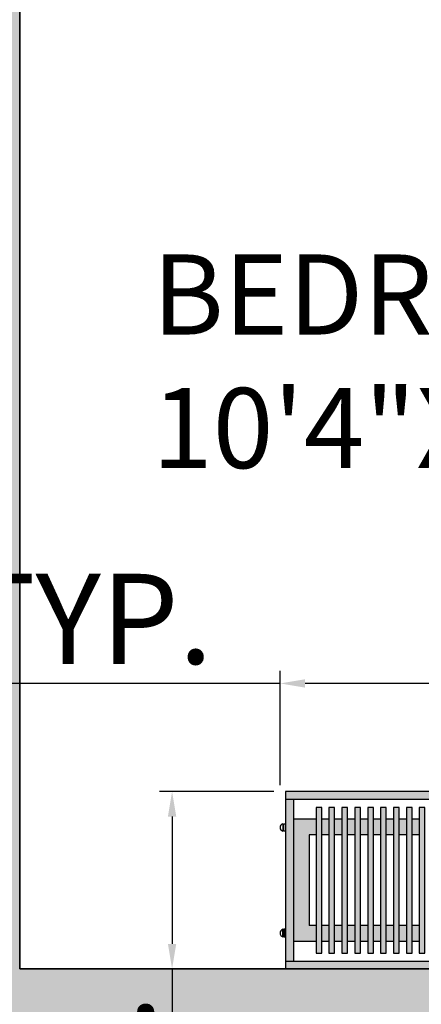
# Model space of a CAD drawing. Units: inches. Extents: x 3592 to 4861, y 1650 to 2243.
# Tile 12 of 30: x 4265 to 4306, y 1772 to 1870. Entities that reach past the tile are written whole.
import ezdxf

# ---------------------------------------------------------------- set-up
doc = ezdxf.new("R2010")
doc.units = ezdxf.units.IN
for name, color, linetype, lineweight in [('A-ANNO-DIMS', 2, 'Continuous', 13), ('A-AREA-IDEN', 7, 'Continuous', 18), ('A-FURN', 9, 'Continuous', 13), ('A-WALL', 7, 'Continuous', 35), ('estofado', 7, 'Continuous', 25)]:
    doc.layers.add(name, color=color, linetype=linetype, lineweight=lineweight)
doc.layers.add('A-WALL-PATT', color=252, linetype='Continuous', lineweight=13, true_color=0x939598)
doc.layers.add('MOBIL', color=7, linetype='Continuous')
doc.styles.get("Standard").update_dxf_attribs({"font": 'arial.ttf'})
doc.dimstyles.new('ISO-25', dxfattribs={"dimtxt": 9, "dimasz": 2.5, "dimexe": 1.25, "dimexo": 0.625, "dimtad": 1, "dimlunit": 3, "dimtxsty": 'Standard', "dimcen": 2.5, "dimadec": 0, "dimazin": 0, "dimtfac": 1, "dimtmove": 0, "dimatfit": 3, "dimfxl": 1, "dimarcsym": 0})

# ---------------------------------------------------------------- blocks, each defined once
blk = doc.blocks.new('Aparador Aido WV')
at = {"layer": 'MOBIL'}
h = blk.add_hatch(color=256, dxfattribs=at)
h.set_gradient(color1=(226, 228, 228), one_color=1, tint=1, name='CYLINDER')
h.paths.add_polyline_path([(0.9, -0.02), (0.9, 0), (-0.9, 0), (-0.9, -0.02)])
h = blk.add_hatch(color=256, dxfattribs=at)
h.set_gradient(color1=(226, 228, 228), one_color=1, tint=1)
h.paths.add_polyline_path([(0.9, -0.02), (0.88, -0.02), (0.88, -0.43), (0.9, -0.43)])
h = blk.add_hatch(color=256, dxfattribs=at)
h.set_gradient(color1=(106, 79, 62), color2=(55, 41, 32), one_color=1, tint=0.17)
h.paths.add_polyline_path([(0.5461, -0.0402), (0.5461, -0.4098), (0.5605, -0.4098), (0.5605, -0.0402)])
h = blk.add_hatch(color=256, dxfattribs=at)
h.set_gradient(color1=(106, 79, 62), color2=(55, 41, 32), one_color=1, tint=0.17)
h.paths.add_polyline_path([(0.5789, -0.0402), (0.5789, -0.4098), (0.5932, -0.4098), (0.5932, -0.0402)])
h = blk.add_hatch(color=256, dxfattribs=at)
h.set_gradient(color1=(106, 79, 62), color2=(55, 41, 32), one_color=1, tint=0.17)
h.paths.add_polyline_path([(0.6116, -0.0402), (0.6116, -0.4098), (0.626, -0.4098), (0.626, -0.0402)])
h = blk.add_hatch(color=256, dxfattribs=at)
h.set_gradient(color1=(106, 79, 62), color2=(55, 41, 32), one_color=1, tint=0.17)
h.paths.add_polyline_path([(0.6444, -0.0402), (0.6444, -0.4098), (0.6587, -0.4098), (0.6587, -0.0402)])
h = blk.add_hatch(color=256, dxfattribs=at)
h.set_gradient(color1=(106, 79, 62), color2=(55, 41, 32), one_color=1, tint=0.17)
h.paths.add_polyline_path([(0.6771, -0.0402), (0.6771, -0.4098), (0.6915, -0.4098), (0.6915, -0.0402)])
h = blk.add_hatch(color=256, dxfattribs=at)
h.set_gradient(color1=(106, 79, 62), color2=(55, 41, 32), one_color=1, tint=0.17)
h.paths.add_polyline_path([(0.7099, -0.0402), (0.7099, -0.4098), (0.7242, -0.4098), (0.7242, -0.0402)])
h = blk.add_hatch(color=256, dxfattribs=at)
h.set_gradient(color1=(106, 79, 62), color2=(55, 41, 32), one_color=1, tint=0.17)
h.paths.add_polyline_path([(0.7426, -0.0402), (0.7426, -0.4098), (0.757, -0.4098), (0.757, -0.0402)])
h = blk.add_hatch(color=256, dxfattribs=at)
h.set_gradient(color1=(106, 79, 62), color2=(55, 41, 32), one_color=1, tint=0.17)
h.paths.add_polyline_path([(0.7754, -0.0402), (0.7754, -0.4098), (0.7897, -0.4098), (0.7897, -0.0402)])
h = blk.add_hatch(color=256, dxfattribs=at)
h.set_gradient(color1=(106, 79, 62), color2=(55, 41, 32), one_color=1, tint=0.17)
h.paths.add_polyline_path([(0.8081, -0.0402), (0.8081, -0.4098), (0.8225, -0.4098), (0.8225, -0.0402)])
h = blk.add_hatch(color=256, dxfattribs=at)
h.set_gradient(color1=(106, 79, 62), color2=(157, 117, 92), one_color=1, tint=0.49)
h.paths.add_polyline_path([(0.5789, -0.07), (0.5605, -0.07), (0.5605, -0.11), (0.5789, -0.11)])
h = blk.add_hatch(color=256, dxfattribs=at)
h.set_gradient(color1=(106, 79, 62), color2=(157, 117, 92), one_color=1, tint=0.49)
h.paths.add_polyline_path([(0.6116, -0.07), (0.5932, -0.07), (0.5932, -0.11), (0.6116, -0.11)])
h = blk.add_hatch(color=256, dxfattribs=at)
h.set_gradient(color1=(106, 79, 62), color2=(157, 117, 92), one_color=1, tint=0.49)
h.paths.add_polyline_path([(0.6444, -0.07), (0.626, -0.07), (0.626, -0.11), (0.6444, -0.11)])
h = blk.add_hatch(color=256, dxfattribs=at)
h.set_gradient(color1=(106, 79, 62), color2=(157, 117, 92), one_color=1, tint=0.49)
h.paths.add_polyline_path([(0.6771, -0.07), (0.6587, -0.07), (0.6587, -0.11), (0.6771, -0.11)])
h = blk.add_hatch(color=256, dxfattribs=at)
h.set_gradient(color1=(106, 79, 62), color2=(157, 117, 92), one_color=1, tint=0.49)
h.paths.add_polyline_path([(0.7099, -0.07), (0.6915, -0.07), (0.6915, -0.11), (0.7099, -0.11)])
h = blk.add_hatch(color=256, dxfattribs=at)
h.set_gradient(color1=(106, 79, 62), color2=(157, 117, 92), one_color=1, tint=0.49)
h.paths.add_polyline_path([(0.7426, -0.07), (0.7242, -0.07), (0.7242, -0.11), (0.7426, -0.11)])
h = blk.add_hatch(color=256, dxfattribs=at)
h.set_gradient(color1=(106, 79, 62), color2=(157, 117, 92), one_color=1, tint=0.49)
h.paths.add_polyline_path([(0.7754, -0.07), (0.757, -0.07), (0.757, -0.11), (0.7754, -0.11)])
h = blk.add_hatch(color=256, dxfattribs=at)
h.set_gradient(color1=(106, 79, 62), color2=(157, 117, 92), one_color=1, tint=0.49)
h.paths.add_polyline_path([(0.8081, -0.07), (0.7897, -0.07), (0.7897, -0.11), (0.8081, -0.11)])
h = blk.add_hatch(color=256, dxfattribs=at)
h.set_gradient(color1=(106, 79, 62), color2=(157, 117, 92), one_color=1, tint=0.49)
h.paths.add_polyline_path([(0.88, -0.07), (0.8225, -0.07), (0.8225, -0.11), (0.84, -0.11), (0.84, -0.34), (0.8225, -0.34), (0.8225, -0.38), (0.88, -0.38)])
h = blk.add_hatch(color=256, dxfattribs=at)
h.set_gradient(color1=(106, 79, 62), color2=(157, 117, 92), one_color=1, tint=0.49)
h.paths.add_polyline_path([(0.5789, -0.34), (0.5605, -0.34), (0.5605, -0.38), (0.5789, -0.38)])
h = blk.add_hatch(color=256, dxfattribs=at)
h.set_gradient(color1=(106, 79, 62), color2=(157, 117, 92), one_color=1, tint=0.49)
h.paths.add_polyline_path([(0.6116, -0.34), (0.5932, -0.34), (0.5932, -0.38), (0.6116, -0.38)])
h = blk.add_hatch(color=256, dxfattribs=at)
h.set_gradient(color1=(106, 79, 62), color2=(157, 117, 92), one_color=1, tint=0.49)
h.paths.add_polyline_path([(0.6444, -0.34), (0.626, -0.34), (0.626, -0.38), (0.6444, -0.38)])
h = blk.add_hatch(color=256, dxfattribs=at)
h.set_gradient(color1=(106, 79, 62), color2=(157, 117, 92), one_color=1, tint=0.49)
h.paths.add_polyline_path([(0.6771, -0.34), (0.6587, -0.34), (0.6587, -0.38), (0.6771, -0.38)])
h = blk.add_hatch(color=256, dxfattribs=at)
h.set_gradient(color1=(106, 79, 62), color2=(157, 117, 92), one_color=1, tint=0.49)
h.paths.add_polyline_path([(0.7099, -0.34), (0.6915, -0.34), (0.6915, -0.38), (0.7099, -0.38)])
h = blk.add_hatch(color=256, dxfattribs=at)
h.set_gradient(color1=(106, 79, 62), color2=(157, 117, 92), one_color=1, tint=0.49)
h.paths.add_polyline_path([(0.7426, -0.34), (0.7242, -0.34), (0.7242, -0.38), (0.7426, -0.38)])
h = blk.add_hatch(color=256, dxfattribs=at)
h.set_gradient(color1=(106, 79, 62), color2=(157, 117, 92), one_color=1, tint=0.49)
h.paths.add_polyline_path([(0.7754, -0.34), (0.757, -0.34), (0.757, -0.38), (0.7754, -0.38)])
h = blk.add_hatch(color=256, dxfattribs=at)
h.set_gradient(color1=(106, 79, 62), color2=(157, 117, 92), one_color=1, tint=0.49)
h.paths.add_polyline_path([(0.8081, -0.34), (0.7897, -0.34), (0.7897, -0.38), (0.8081, -0.38)])
h = blk.add_hatch(color=256, dxfattribs=at)
h.set_gradient(color1=(226, 228, 228), one_color=1, tint=1, name='CYLINDER')
h.paths.add_polyline_path([(0.9, -0.45), (0.9, -0.43), (-0.9, -0.43), (-0.9, -0.45)])
at = {"layer": 'estofado', "ltscale": 0.5}
for p, q in [((0.5605, -0.07), (0.5789, -0.07)), ((0.5932, -0.07), (0.6116, -0.07)), ((0.626, -0.07), (0.6444, -0.07)), ((0.6587, -0.07), (0.6771, -0.07)), ((0.6915, -0.07), (0.7099, -0.07)), ((0.7242, -0.07), (0.7426, -0.07)), ((0.757, -0.07), (0.7754, -0.07)), ((0.7897, -0.07), (0.8081, -0.07)), ((0.8225, -0.07), (0.88, -0.07)), ((0.9067, -0.0817), (0.9067, -0.1006)), ((0.5605, -0.11), (0.5789, -0.11)), ((0.5932, -0.11), (0.6116, -0.11)), ((0.626, -0.11), (0.6444, -0.11)), ((0.6587, -0.11), (0.6771, -0.11)), ((0.6915, -0.11), (0.7099, -0.11)), ((0.7242, -0.11), (0.7426, -0.11)), ((0.757, -0.11), (0.7754, -0.11)), ((0.7897, -0.11), (0.8081, -0.11)), ((0.8225, -0.11), (0.84, -0.11)), ((0.84, -0.34), (0.84, -0.11)), ((0.5605, -0.34), (0.5789, -0.34)), ((0.5932, -0.34), (0.6116, -0.34)), ((0.626, -0.34), (0.6444, -0.34)), ((0.6587, -0.34), (0.6771, -0.34)), ((0.6915, -0.34), (0.7099, -0.34)), ((0.7242, -0.34), (0.7426, -0.34)), ((0.757, -0.34), (0.7754, -0.34)), ((0.7897, -0.34), (0.8081, -0.34)), ((0.8225, -0.34), (0.84, -0.34)), ((0.9067, -0.3683), (0.9067, -0.3494)), ((0.5605, -0.38), (0.5789, -0.38)), ((0.5932, -0.38), (0.6116, -0.38)), ((0.626, -0.38), (0.6444, -0.38)), ((0.6587, -0.38), (0.6771, -0.38)), ((0.6915, -0.38), (0.7099, -0.38)), ((0.7242, -0.38), (0.7426, -0.38)), ((0.757, -0.38), (0.7754, -0.38)), ((0.7897, -0.38), (0.8081, -0.38)), ((0.8225, -0.38), (0.88, -0.38))]:
    blk.add_line(p, q, dxfattribs=at)
for points in [[(0.5461, -0.0402), (0.5461, -0.4098), (0.5605, -0.4098), (0.5605, -0.0402)], [(0.5789, -0.0402), (0.5789, -0.4098), (0.5932, -0.4098), (0.5932, -0.0402)], [(0.6116, -0.0402), (0.6116, -0.4098), (0.626, -0.4098), (0.626, -0.0402)], [(0.6444, -0.0402), (0.6444, -0.4098), (0.6587, -0.4098), (0.6587, -0.0402)], [(0.6771, -0.0402), (0.6771, -0.4098), (0.6915, -0.4098), (0.6915, -0.0402)], [(0.7099, -0.0402), (0.7099, -0.4098), (0.7242, -0.4098), (0.7242, -0.0402)], [(0.7426, -0.0402), (0.7426, -0.4098), (0.757, -0.4098), (0.757, -0.0402)], [(0.7754, -0.0402), (0.7754, -0.4098), (0.7897, -0.4098), (0.7897, -0.0402)], [(0.8081, -0.0402), (0.8081, -0.4098), (0.8225, -0.4098), (0.8225, -0.0402)], [(0.9054, -0.0817), (0.9009, -0.0817), (0.9009, -0.1006), (0.9054, -0.1006)], [(0.9054, -0.3683), (0.9009, -0.3683), (0.9009, -0.3494), (0.9054, -0.3494)]]:
    blk.add_lwpolyline(points, close=True, dxfattribs=at)
for centre in [(0.904, -0.0911), (0.904, -0.3589)]:
    blk.add_arc(centre, 0.0098, 285.9849, 74.0151, dxfattribs=at)
at = {"layer": 'MOBIL'}
for p, q in [((0.9, -0.02), (-0.9, -0.02)), ((0.88, -0.43), (0.88, -0.02)), ((-0.9, -0.43), (0.9, -0.43))]:
    blk.add_line(p, q, dxfattribs=at)
blk.add_lwpolyline([(-0.9, -0.45), (0.9, -0.45), (0.9, 0), (-0.9, 0)], close=True, dxfattribs=at)
blk = doc.blocks.new('*D156')
at = {"layer": 'A-ANNO-DIMS', "color": 0, "lineweight": -2, "transparency": 16777216}
for p, q in [((4291.393, 1793.561), (4291.393, 1804.979)), ((4363.347, 1793.561), (4363.347, 1804.979)), ((4291.393, 1803.729), (4155.277, 1803.729)), ((4360.847, 1803.729), (4293.893, 1803.729))]:
    blk.add_line(p, q, dxfattribs=at)
at = {"layer": 'A-ANNO-DIMS', "color": 0, "transparency": 16777216}
for points in [[(4293.893, 1804.145), (4293.893, 1803.312), (4291.393, 1803.729)], [(4360.847, 1804.145), (4360.847, 1803.312), (4363.347, 1803.729)]]:
    blk.add_solid(points, dxfattribs=at)
at = {"layer": 'Defpoints', "color": 0, "transparency": 16777216}
for p in [(4291.393, 1803.729), (4291.393, 1792.936), (4363.347, 1792.936)]:
    blk.add_point(p, dxfattribs=at)
at = {"layer": 'A-ANNO-DIMS', "color": 0, "transparency": 16777216, "insert": (4222.085, 1809.01), "char_height": 9, "attachment_point": 5}
blk.add_mtext('SIDEBOARD 6\'-0" TYP.', dxfattribs=at)
blk = doc.blocks.new('*D157')
at = {"layer": 'A-ANNO-DIMS', "color": 0, "lineweight": -2, "transparency": 16777216}
for p, q in [((4290.768, 1792.936), (4279.35, 1792.936)), ((4280.6, 1790.436), (4280.6, 1777.719)), ((4290.768, 1775.219), (4279.35, 1775.219)), ((4280.6, 1775.219), (4280.6, 1696.485))]:
    blk.add_line(p, q, dxfattribs=at)
at = {"layer": 'A-ANNO-DIMS', "color": 0, "transparency": 16777216}
for points in [[(4280.183, 1790.436), (4281.016, 1790.436), (4280.6, 1792.936)], [(4280.183, 1777.719), (4281.016, 1777.719), (4280.6, 1775.219)]]:
    blk.add_solid(points, dxfattribs=at)
at = {"layer": 'Defpoints', "color": 0, "transparency": 16777216}
for p in [(4291.393, 1792.936), (4280.6, 1775.219), (4291.393, 1775.219)]:
    blk.add_point(p, dxfattribs=at)
at = {"layer": 'A-ANNO-DIMS', "color": 0, "transparency": 16777216, "insert": (4275.321, 1734.602), "char_height": 9, "attachment_point": 5, "rotation": 90}
blk.add_mtext('1\'-5 1/2" TYP.', dxfattribs=at)

msp = doc.modelspace()

# ---------------------------------------------------------------- hatches: boundary and pattern name
at = {"layer": 'A-WALL-PATT'}
h = msp.add_hatch(color=256, dxfattribs=at)
h.dxf.hatch_style = 1
h.paths.add_polyline_path([(4398.37, 2165.219), (4038.37, 2165.219), (4038.37, 1993.219), (4047.37, 1993.219), (4047.37, 2156.219), (4191.37, 2156.219), (4191.37, 2150.219), (4195.37, 2150.219), (4195.37, 2156.219), (4256.37, 2156.219), (4256.37, 2150.219), (4265.37, 2150.219), (4265.37, 2156.219), (4389.37, 2156.219), (4389.37, 2114.219), (4398.37, 2114.219)])
h.paths.add_polyline_path([(4265.37, 2102.219), (4256.37, 2102.219), (4256.37, 2096.219), (4195.37, 2096.219), (4195.37, 2102.219), (4191.37, 2102.219), (4191.37, 2020.219), (4195.37, 2020.219), (4195.37, 2087.219), (4256.37, 2087.219), (4256.37, 2020.219), (4306.37, 2020.219), (4306.37, 2024.219), (4265.37, 2024.219)], flags=17)
h.paths.add_polyline_path([(4398.37, 2066.219), (4389.37, 2066.219), (4389.37, 2024.219), (4348.37, 2024.219), (4348.37, 2020.219), (4389.37, 2020.219), (4389.37, 1989.719), (4398.37, 1989.719)])
h.paths.add_polyline_path([(4398.37, 1941.719), (4389.37, 1941.719), (4389.37, 1911.219), (4301.37, 1911.219), (4301.37, 1907.219), (4389.37, 1907.219), (4389.37, 1865.219), (4398.37, 1865.219)])
h.paths.add_polyline_path([(4398.37, 1817.219), (4389.37, 1817.219), (4389.37, 1775.219), (4265.37, 1775.219), (4265.37, 1911.219), (4256.37, 1911.219), (4256.37, 1817.219), (4220.87, 1817.219), (4220.87, 1808.219), (4256.37, 1808.219), (4256.37, 1766.219), (4389.37, 1766.219), (4389.37, 1694.219), (4256.37, 1694.219), (4256.37, 1685.219), (4398.37, 1685.219)])
h.paths.add_polyline_path([(4178.87, 1817.219), (4077.37, 1817.219), (4077.37, 1808.219), (4178.87, 1808.219)])
h.paths.add_polyline_path([(4111.37, 2020.219), (4155.37, 2020.219), (4155.37, 2024.219), (4077.37, 2024.219), (4077.37, 2020.219), (4107.37, 2020.219), (4107.37, 1942.219), (4047.37, 1942.219), (4047.37, 1969.219), (4038.37, 1969.219), (4038.37, 1911.219), (4047.37, 1911.219), (4047.37, 1938.219), (4107.37, 1938.219), (4107.37, 1860.219), (4077.37, 1860.219), (4077.37, 1856.219), (4111.37, 1856.219)])
h.paths.add_polyline_path([(4047.37, 1887.219), (4038.37, 1887.219), (4038.37, 1685.219), (4152.37, 1685.219), (4152.37, 1715.219), (4143.37, 1715.219), (4143.37, 1694.219), (4047.37, 1694.219)])
h.paths.add_polyline_path([(4152.37, 1772.219), (4143.37, 1772.219), (4143.37, 1751.219), (4152.37, 1751.219)], flags=17)

# ---------------------------------------------------------------- linework, layer by layer
at = {"layer": 'A-WALL'}
for p in [(4265.37, 1911.219), (4389.37, 1775.219)]:
    msp.add_line(p, (4265.37, 1775.219), dxfattribs=at)

# ---------------------------------------------------------------- block references
at = {"layer": 'A-FURN', "xscale": 39.3701, "yscale": 39.3701, "zscale": 39.3701, "rotation": 180}
msp.add_blockref('Aparador Aido WV', (4327.37, 1775.219), dxfattribs=at)

# ---------------------------------------------------------------- texts
at = {"layer": 'A-AREA-IDEN', "insert": (4278.607, 1846.565), "char_height": 8, "attachment_point": 1}
msp.add_mtext_dynamic_manual_height_columns('BEDROOM\\P10\'4"X11\'0"', width=121.44943, gutter_width=12.5, heights=[0], dxfattribs=at)

# ---------------------------------------------------------------- dimensions: what is measured, and where the dimension line sits
at = {"layer": 'A-ANNO-DIMS'}
for base, p1, p2, angle, text, picture, middle in [((4291.393, 1803.729), (4363.347, 1792.936), (4291.393, 1792.936), 180, 'SIDEBOARD <> TYP.', '*D156', (4222.085, 1809.01)), ((4280.6, 1775.219), (4291.393, 1792.936), (4291.393, 1775.219), 270, '<> TYP.', '*D157', (4275.321, 1734.602))]:
    dim = msp.add_linear_dim(base=base, p1=p1, p2=p2, angle=angle, text=text, dimstyle='ISO-25', override={"dimdec": 1, "dimlfac": 1, "dimrnd": 0, "dimzin": 1, "dimdsep": 46, "dimlunit": 4, "dimfrac": 2}, dxfattribs=at)
    dim.commit()
    dim.dimension.update_dxf_attribs({"geometry": picture, "text_midpoint": middle})

doc.saveas('drawing.dxf')
